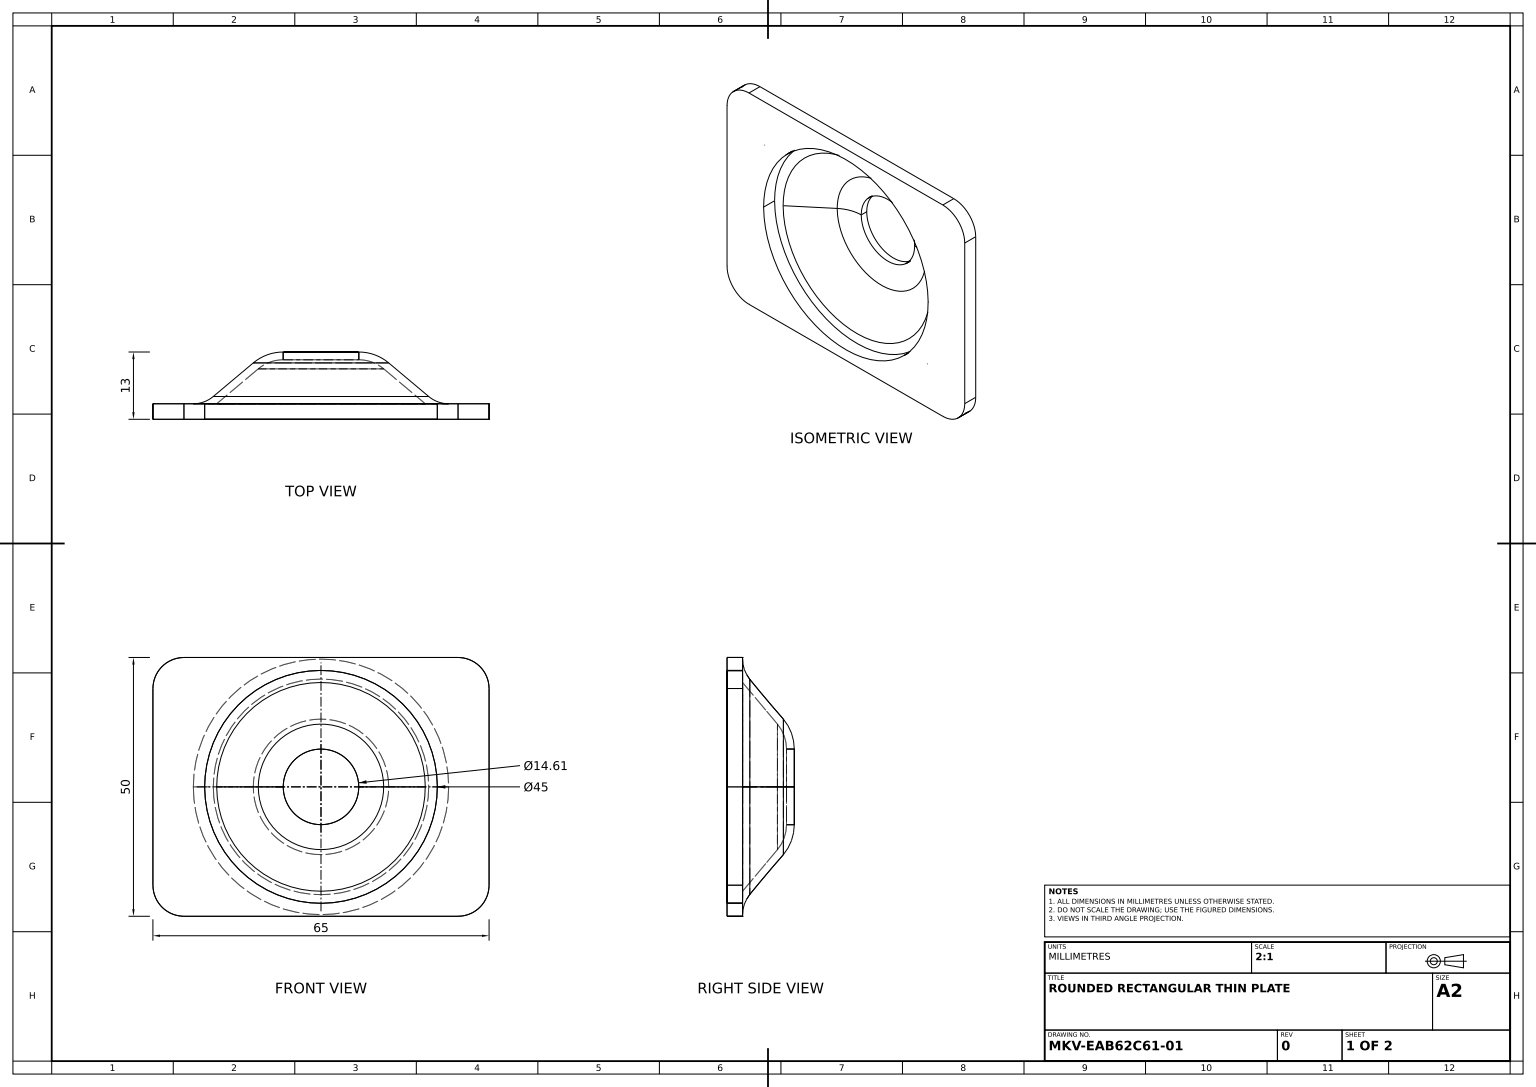
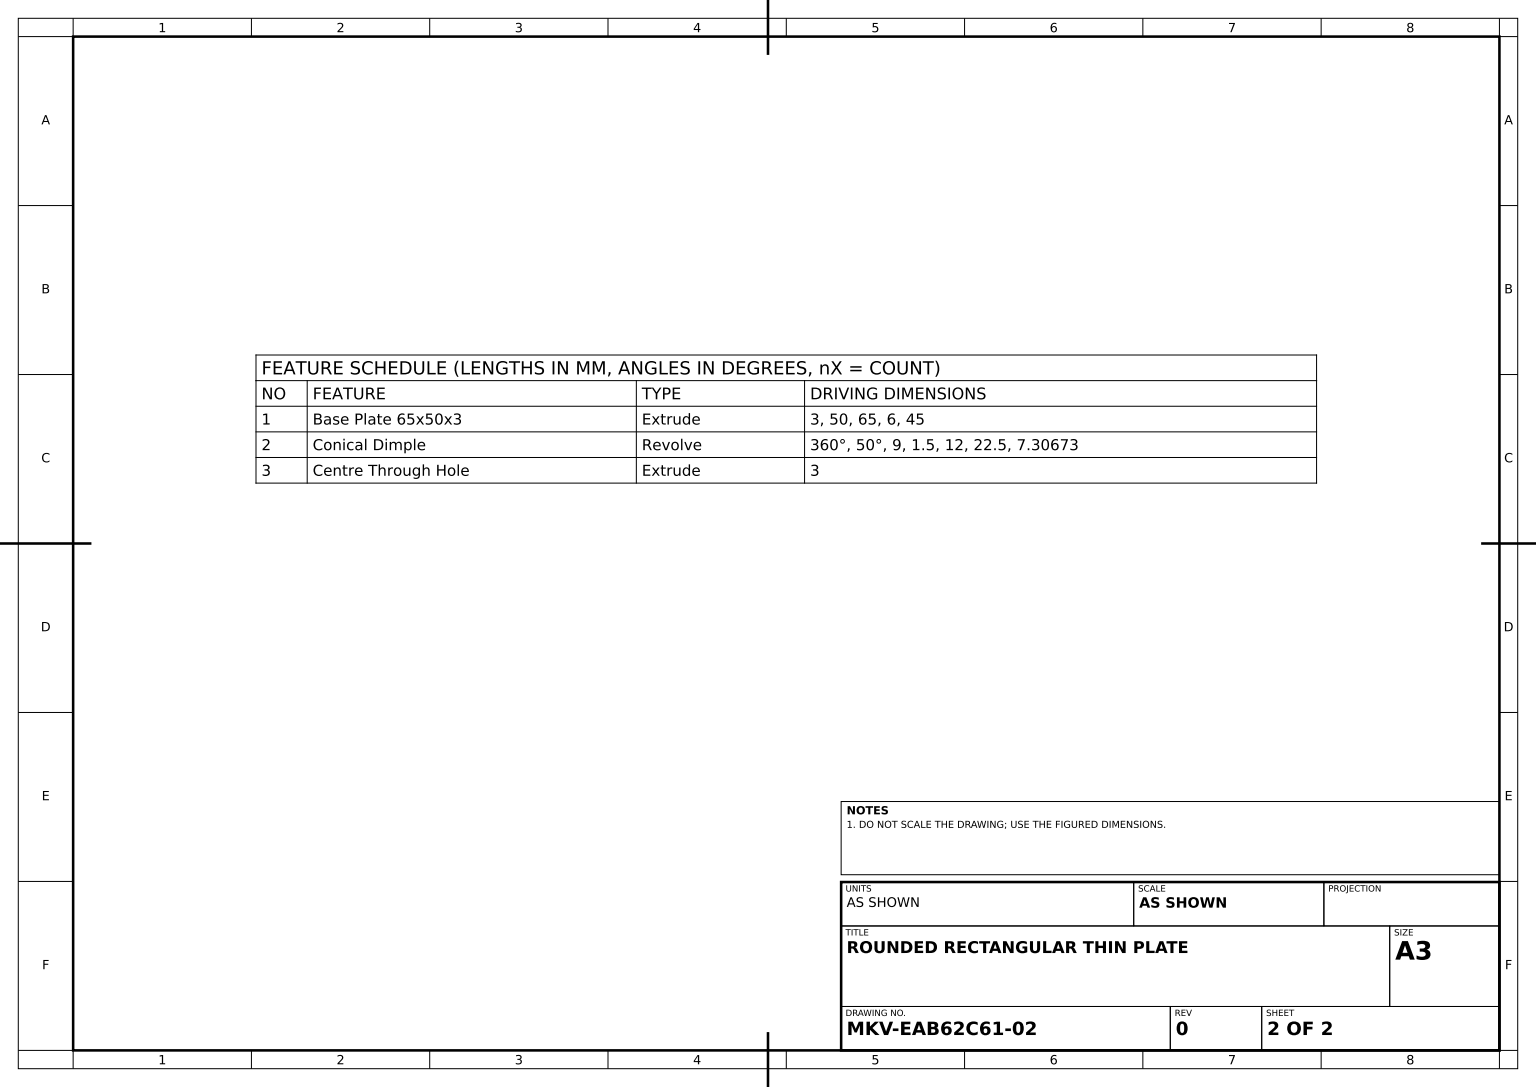
from build123d import *

# Parameters (mm, degrees)
PLATE_PROFILE_SKETCH_R    = 22.5
BASE_PLATE_65X50X3_DEPTH  = 3
CENTRE_HOLE_SKETCH_R      = 7.306731966
CENTRE_THROUGH_HOLE_DEPTH = 3


with BuildPart() as part:
    # Plate Profile Sketch → Base Plate 65x50x3 (new body)
    with BuildSketch(Plane.XY):
        with BuildLine():
            Line((-26.5, -25), (26.5, -25))
            ThreePointArc((26.5, -25), (30.742640687, -23.242640687), (32.5, -19))
            Line((32.5, -19), (32.5, 19))
            ThreePointArc((32.5, 19), (30.742640687, 23.242640687), (26.5, 25))
            Line((26.5, 25), (-26.5, 25))
            ThreePointArc((-26.5, 25), (-30.742640687, 23.242640687), (-32.5, 19))
            Line((-32.5, 19), (-32.5, -19))
            ThreePointArc((-32.5, -19), (-30.742640687, -23.242640687), (-26.5, -25))
        make_face()
        Circle(PLATE_PROFILE_SKETCH_R, mode=Mode.SUBTRACT)
    extrude(amount=BASE_PLATE_65X50X3_DEPTH)

    # Conical Dimple Profile Sketch → Conical Dimple (revolve)
    with BuildSketch(Plane(origin=(0, 0, 0), x_dir=(1, 0, 0), z_dir=(0, 1, 0))):
        with BuildLine():
            Line((13.091820453, 7.894399988), (20.827095747, 1.403733341))
            ThreePointArc((20.827095747, 1.403733341), (22.631700546, 0.361844275), (24.683821406, 0))
            Line((24.683821406, 0), (20.16641426, 0))
            Line((20.16641426, 0), (12.127639038, 6.745333323))
            ThreePointArc((12.127639038, 6.745333323), (9.871883041, 8.047694656), (7.306731966, 8.5))
            Line((7.306731966, 8.5), (0, 8.5))
            Line((0, 8.5), (0, 10))
            Line((0, 10), (7.306731966, 10))
            ThreePointArc((7.306731966, 10), (10.384913256, 9.457233587), (13.091820453, 7.894399988))
        make_face()
    revolve(axis=Axis((0, 0, 5.787775716), (0, 0, -1)))

    # Centre Hole Sketch → Centre Through Hole (cut)
    with BuildSketch(Plane(origin=(0, 0, -10), x_dir=(-1, 0, 0), z_dir=(0, 0, -1))):
        with Locations(Location((0, 0, 0), (0, 0, 180))):
            Circle(CENTRE_HOLE_SKETCH_R)
    extrude(amount=-CENTRE_THROUGH_HOLE_DEPTH, mode=Mode.SUBTRACT)


solid = part.part
